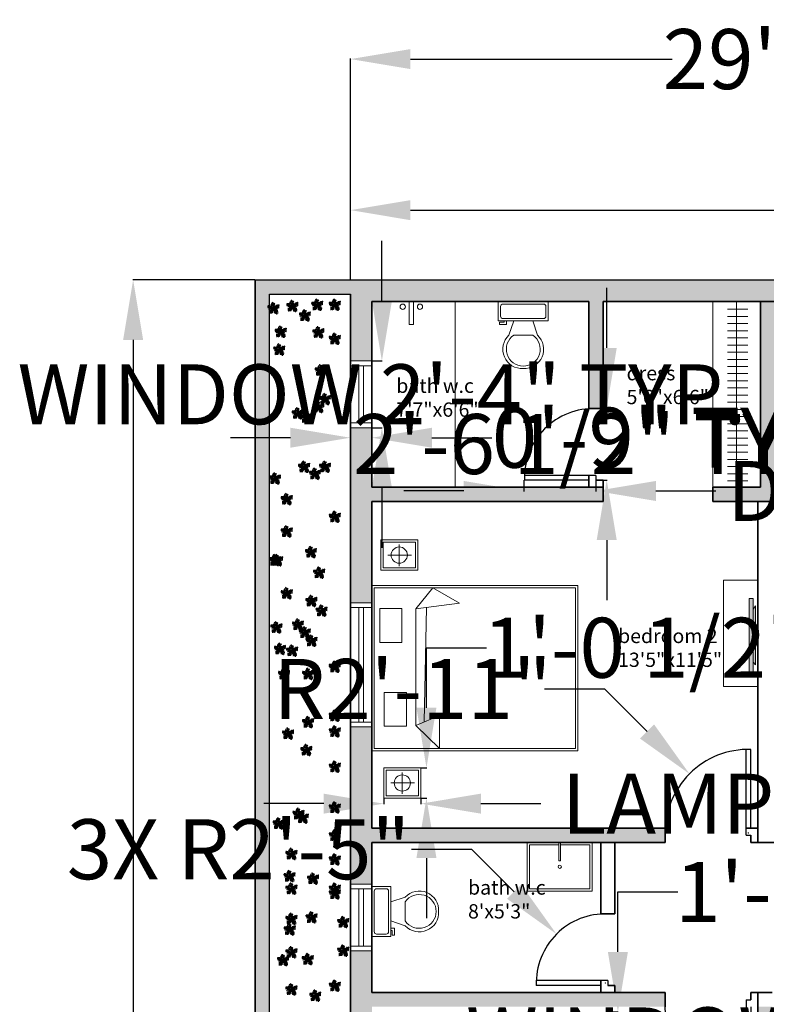
# Model space of a CAD drawing. Units: inches. Extents: x 23 to 3024, y 4 to 1405.
# Tile 2 of 7: x 2062 to 2375, y 992 to 1405. Entities that reach past the tile are written whole.
import ezdxf

# ---------------------------------------------------------------- set-up
doc = ezdxf.new("R2010")
doc.units = ezdxf.units.IN
doc.header["$MEASUREMENT"] = 0
for name, color, linetype, lineweight in [('A-ANNO-DIMS', 2, 'Continuous', 18), ('A-DOOR', 4, 'Continuous', 25), ('A-EQPM', 8, 'Continuous', 18), ('A-EQPM-PATT', 7, 'Continuous', 13), ('A-FLOR-CASE', 9, 'Continuous', 18), ('A-FLOR-FIXT', 9, 'Continuous', 18), ('A-WALL', 7, 'Continuous', 35), ('A-WALL-PATT', 189, 'Continuous', 13), ('C-PROP', 7, 'Continuous', 30), ('L-PLNT', 114, 'Continuous', 13)]:
    doc.layers.add(name, color=color, linetype=linetype, lineweight=lineweight)
for name, color, linetype, lineweight, true_color in [('A-AREA-IDEN', 30, 'Continuous', 18, 0xf8991e), ('A-FURN', 141, 'Continuous', 18, 0xadddf7), ('A-GLAZ', 30, 'Continuous', 18, 0xf26722)]:
    doc.layers.add(name, color=color, linetype=linetype, lineweight=lineweight, true_color=true_color)
doc.styles.get("Standard").update_dxf_attribs({"font": 'arial.ttf'})
doc.dimstyles.get("Standard").update_dxf_attribs({"dimtxt": 25.18, "dimasz": 25.18, "dimexe": 0.18, "dimexo": 0.0625, "dimgap": 0.09, "dimtad": 0, "dimtih": 1, "dimtoh": 1, "dimdec": 0, "dimrnd": 10, "dimzin": 0, "dimdsep": 46, "dimlunit": 3, "dimtxsty": 'Standard', "dimcen": 0.09, "dimadec": 0, "dimazin": 0, "dimtfac": 1, "dimtdec": 0, "dimtofl": 0, "dimtmove": 0, "dimatfit": 3, "dimfxl": 1, "dimtolj": 1, "dimtzin": 0, "dimarcsym": 0})

# ---------------------------------------------------------------- blocks, each defined once
blk = doc.blocks.new('*U2')
for p, q in [((9.5, -6), (9.5, -2)), ((-8, -8.5), (-8, -8)), ((-7, -8), (-7, -9.5)), ((-4, -8), (-6, -14)), ((4, -8), (6, -14)), ((-10, -8.5), (-8, -8.5)), ((-10, -9.5), (-10, -8.5)), ((-7, -9.5), (-10, -9.5)), ((4, -14), (-4, -14))]:
    blk.add_line(p, q)
blk.add_lwpolyline([(10.5, -8), (10.5, 0), (-10.5, 0), (-10.5, -8)], close=True)
for points in [[(-9.5, -2), (-9.5, -6)], [(8.5, -1), (-8.5, -1)], [(-8.5, -7), (8.5, -7)]]:
    blk.add_lwpolyline(points)
for centre, radius, start, end in [((-8.625, -1.875), 0.8839, 81.8699, 188.1301), ((8.625, -1.875), 0.8839, 351.8699, 98.1301), ((-8.625, -6.125), 0.8839, 171.869898, 278.1301), ((8.625, -6.125), 0.8839, 261.8699, 8.1301), ((-0.4772, -19.9188), 8.0953, 133.01722, 273.38), ((0.0374, -19.8731), 7.127, 124.50543, 269.7), ((-0.0373, -19.8731), 7.127, 270.3, 55.4946), ((0.4773, -19.9188), 8.0953, 266.62, 46.9828)]:
    blk.add_arc(centre, radius, start, end)
blk = doc.blocks.new('*U8')
for p, q in [((-47.498, 19.737), (-55.83, 18.344)), ((-40.615, 13.7), (-55.105, 10.913)), ((-31.5, 4.5), (-52.5, 25.5)), ((-33.37, 6.269), (-52.207, 5.34)), ((-48.585, 21.131), (-49.309, 29.026)), ((-28.299, 3.483), (-47.86, -5.805)), ((-43.513, 28.561), (-42.427, 15.558)), ((-38.442, 26.239), (-34.819, 7.663)), ((-21.416, 3.018), (-38.079, -8.128)), ((-35.544, 28.097), (-24.314, 3.947)), ((0, 0), (-31.5, 4.5)), ((-14.533, 2.09), (-30.834, 25.31)), ((-15.982, 2.09), (-30.11, -9.521)), ((-3.665, 19.273), (-27.574, 35.527)), ((-5.114, 28.097), (-24.676, 40.636)), ((-24.314, 23.917), (-2.941, 13.7)), ((0, 0), (-22.5, -19.5)), ((-7.288, 39.707), (-21.778, 46.673)), ((-6.563, 1.161), (-21.416, -8.128)), ((-20.691, 13.7), (-1.129, 4.876)), ((-8.737, 47.138), (-17.069, 52.711)), ((-10.186, 53.64), (-13.084, 55.962)), ((0, 0), (-10.5, 57)), ((-9.099, 51.782), (-6.563, 55.962)), ((-7.65, 43.423), (-2.578, 49.46)), ((-5.839, 35.992), (4.667, 48.067)), ((-5.114, 27.632), (10.463, 46.673)), ((-2.941, 16.486), (8.652, 37.85)), ((-1.129, 6.734), (9.014, 26.704)), ((0, 0), (27, 9)), ((0, 0), (18, -22.5)), ((3.942, 1.625), (11.187, 24.381)), ((6.478, 1.625), (26.04, -8.592)), ((10.101, 3.483), (17.708, 26.239)), ((11.187, 3.483), (30.749, -5.805)), ((16.259, 5.805), (23.142, 31.348)), ((18.07, 5.805), (35.096, -3.483)), ((22.055, 7.198), (27.489, 32.277)), ((24.229, 7.663), (46.688, 1.625)), ((27, 9), (48, 36)), ((27.127, 9.056), (31.112, 35.992)), ((29.662, 12.307), (48.137, 6.269)), ((31.836, 30.883), (32.561, 16.486)), ((33.285, 16.486), (48.862, 10.913)), ((35.096, 32.741), (37.27, 22.524)), ((36.183, 19.737), (48.137, 17.88)), ((38.719, 34.134), (41.979, 28.561)), ((40.53, 25.775), (48.862, 24.846)), ((43.791, 29.954), (51.036, 30.883)), ((44.153, 36.456), (45.239, 32.741)), ((-17.431, -15.094), (-42.789, -18.809)), ((-28.299, -29.026), (-42.789, -31.348)), ((-24.314, -21.596), (-42.427, -22.06)), ((-30.834, -34.135), (-42.427, -35.528)), ((-34.457, -39.708), (-40.978, -42.494)), ((-26.849, -26.24), (-40.253, -25.775)), ((-22.5, -19.5), (-37.5, -45)), ((-32.646, -36.921), (-31.921, -44.352)), ((-15.257, -12.772), (-30.11, -12.772)), ((-29.023, -30.884), (-27.936, -43.887)), ((-25.038, -23.918), (-22.865, -45.281)), ((-20.691, -18.345), (-17.793, -44.352)), ((-6.563, -5.805), (-19.967, -9.985)), ((-17.069, -15.094), (-12.721, -40.172)), ((-13.446, -11.378), (-8.737, -32.741)), ((-9.461, -8.592), (-6.201, -23.453)), ((-4.752, -3.483), (-3.665, -14.629)), ((2.493, -3.019), (-1.491, -20.202)), ((1.769, -2.555), (24.229, -9.521)), ((5.029, -6.27), (2.131, -25.775)), ((9.014, -11.378), (3.58, -35.992)), ((14.085, -16.951), (6.478, -40.172)), ((7.565, -9.056), (32.198, -14.629)), ((18.07, -22.524), (8.289, -45.745)), ((12.274, -15.094), (36.907, -18.809)), ((20.244, -30.419), (15.897, -44.816)), ((16.259, -19.738), (36.183, -22.989)), ((18, -22.5), (27, -52.5)), ((18.433, -22.524), (40.53, -29.026)), ((19.157, -25.311), (38.719, -33.206)), ((22.78, -37.85), (19.519, -48.532)), ((21.331, -32.741), (39.081, -40.636)), ((22.78, -38.314), (34.372, -44.816)), ((24.591, -45.745), (23.142, -50.854)), ((24.591, -43.423), (30.749, -47.603)), ((26.764, -49.925), (28.213, -50.854))]:
    blk.add_line(p, q)
blk = doc.blocks.new('*D9')
at = {"layer": 'A-ANNO-DIMS', "color": 0, "lineweight": -2, "transparency": 16777216}
for p, q in [((2200.45, 1295.99), (2200.45, 1325.4)), ((2225.63, 1325.22), (2478.99, 1325.22)), ((2775.27, 1325.22), (2521.91, 1325.22)), ((2800.45, 1295.99), (2800.45, 1325.4))]:
    blk.add_line(p, q, dxfattribs=at)
at = {"layer": 'A-ANNO-DIMS', "color": 0, "transparency": 16777216}
for points in [[(2225.63, 1329.42), (2225.63, 1321.02), (2200.45, 1325.22)], [(2775.27, 1329.42), (2775.27, 1321.02), (2800.45, 1325.22)]]:
    blk.add_solid(points, dxfattribs=at)
at = {"layer": 'Defpoints', "color": 0, "transparency": 16777216}
for p in [(2800.45, 1325.22), (2200.45, 1295.93), (2800.45, 1295.93)]:
    blk.add_point(p, dxfattribs=at)
at = {"layer": 'A-ANNO-DIMS', "color": 0, "transparency": 16777216, "insert": (2500.45, 1325.22), "char_height": 25.18, "attachment_point": 5}
blk.add_mtext("\\A1;50'", dxfattribs=at)
blk = doc.blocks.new('*D10')
at = {"layer": 'A-ANNO-DIMS', "color": 0, "lineweight": -2, "transparency": 16777216}
for p, q in [((2160.39, 1295.93), (2109.1, 1295.93)), ((2109.28, 1270.75), (2109.28, 948.87)), ((2109.28, 601.11), (2109.28, 922.98)), ((2160.39, 575.93), (2109.1, 575.93))]:
    blk.add_line(p, q, dxfattribs=at)
at = {"layer": 'A-ANNO-DIMS', "color": 0, "transparency": 16777216}
for points in [[(2105.08, 1270.75), (2113.48, 1270.75), (2109.28, 1295.93)], [(2105.08, 601.11), (2113.48, 601.11), (2109.28, 575.93)]]:
    blk.add_solid(points, dxfattribs=at)
at = {"layer": 'Defpoints', "color": 0, "transparency": 16777216}
for p in [(2160.45, 1295.93), (2109.28, 575.93), (2160.45, 575.93)]:
    blk.add_point(p, dxfattribs=at)
at = {"layer": 'A-ANNO-DIMS', "color": 0, "transparency": 16777216, "insert": (2109.28, 935.93), "char_height": 25.18, "attachment_point": 5}
blk.add_mtext("\\A1;60'", dxfattribs=at)
blk = doc.blocks.new('DOOR-SWING-36IN')
for p, q in [((-1, -1), (-1, 35)), ((1, 2), (1, 35)), ((-1, -1), (1, -1))]:
    blk.add_line(p, q)
blk.add_arc((0, 0), 35.01, 88.3634, 181.6366)
blk = doc.blocks.new('DOOR-SWING-30IN')
for p, q in [((1, 1), (-29, 1)), ((1, 1), (1, -1)), ((-2, -1), (-29, -1))]:
    blk.add_line(p, q)
blk.add_arc((0, 0), 29.02, 88.0251, 181.9749)
blk = doc.blocks.new('WINDOW-48IN')
for p, q in [((9, 52), (0, 52)), ((9, 50), (0, 50)), ((3.5, 2), (3.5, 50)), ((5.5, 2), (5.5, 50)), ((9, 2), (0, 2)), ((9, 0), (0, 0))]:
    blk.add_line(p, q)
blk = doc.blocks.new('WINDOW-24IN')
for p, q in [((9, 28), (0, 28)), ((9, 26), (0, 26)), ((3.5, 2), (3.5, 26)), ((5.5, 2), (5.5, 26)), ((9, 2), (0, 2)), ((9, 0), (0, 0))]:
    blk.add_line(p, q)
blk = doc.blocks.new('NIGHTSTAND-LAMP')
for p, q in [((7.79, 10.75), (7.79, 1.76)), ((2.95, 6.35), (12.92, 6.35))]:
    blk.add_line(p, q)
for points in [[(0, 12.71), (15.59, 12.71), (15.59, 0), (0, 0)], [(1, 11.71), (14.59, 11.71), (14.59, 1), (1, 1)]]:
    blk.add_lwpolyline(points, close=True)
blk.add_circle((7.79, 6.35), 3.4)
blk = doc.blocks.new('*D25')
at = {"layer": 'A-ANNO-DIMS', "color": 0, "lineweight": -2, "transparency": 16777216}
for p, q in [((2273.17, 1211.86), (2273.17, 1207.21)), ((2303.45, 1211.86), (2303.45, 1207.21)), ((2247.99, 1207.39), (2222.81, 1207.39)), ((2328.63, 1207.39), (2353.81, 1207.39))]:
    blk.add_line(p, q, dxfattribs=at)
at = {"layer": 'A-ANNO-DIMS', "color": 0, "transparency": 16777216}
for points in [[(2247.99, 1211.58), (2247.99, 1203.19), (2273.17, 1207.39)], [(2328.63, 1211.58), (2328.63, 1203.19), (2303.45, 1207.39)]]:
    blk.add_solid(points, dxfattribs=at)
at = {"layer": 'Defpoints', "color": 0, "transparency": 16777216}
for p in [(2273.17, 1211.93), (2303.45, 1211.93), (2303.45, 1207.39)]:
    blk.add_point(p, dxfattribs=at)
at = {"layer": 'A-ANNO-DIMS', "color": 0, "transparency": 16777216, "insert": (2517, 1207.39), "char_height": 25.18, "attachment_point": 5}
blk.add_mtext('\\A1;DOOR 2\'-6 1/2" TYP.', dxfattribs=at)
blk = doc.blocks.new('*D26')
at = {"layer": 'A-ANNO-DIMS', "color": 0, "lineweight": -2, "transparency": 16777216}
for p, q in [((2307.99, 1267.38), (2307.99, 1292.56)), ((2303.51, 1242.2), (2308.17, 1242.2)), ((2303.51, 1211.93), (2308.17, 1211.93)), ((2307.99, 1186.75), (2307.99, 1161.57))]:
    blk.add_line(p, q, dxfattribs=at)
at = {"layer": 'A-ANNO-DIMS', "color": 0, "transparency": 16777216}
for points in [[(2303.79, 1267.38), (2312.19, 1267.38), (2307.99, 1242.2)], [(2303.79, 1186.75), (2312.19, 1186.75), (2307.99, 1211.93)]]:
    blk.add_solid(points, dxfattribs=at)
at = {"layer": 'Defpoints', "color": 0, "transparency": 16777216}
for p in [(2303.45, 1242.2), (2307.99, 1242.2), (2303.45, 1211.93)]:
    blk.add_point(p, dxfattribs=at)
at = {"layer": 'A-ANNO-DIMS', "color": 0, "transparency": 16777216, "insert": (2307.99, 1227.07), "char_height": 25.18, "attachment_point": 5}
blk.add_mtext('\\A1;2\'-6 1/2" TYP.', dxfattribs=at)
blk = doc.blocks.new('*D27')
at = {"layer": 'A-ANNO-DIMS', "color": 0, "lineweight": -2, "transparency": 16777216}
for p, q in [((2217.25, 952.93), (2217.25, 978.11)), ((2217.25, 978.11), (2242.43, 978.11)), ((2209.51, 952.93), (2217.43, 952.93)), ((2217.25, 926.11), (2217.25, 927.75)), ((2209.51, 900.93), (2217.43, 900.93))]:
    blk.add_line(p, q, dxfattribs=at)
at = {"layer": 'A-ANNO-DIMS', "color": 0, "transparency": 16777216}
for points in [[(2213.05, 927.75), (2221.45, 927.75), (2217.25, 952.93)], [(2213.05, 926.11), (2221.45, 926.11), (2217.25, 900.93)]]:
    blk.add_solid(points, dxfattribs=at)
at = {"layer": 'Defpoints', "color": 0, "transparency": 16777216}
for p in [(2209.45, 952.93), (2217.25, 952.93), (2209.45, 900.93)]:
    blk.add_point(p, dxfattribs=at)
at = {"layer": 'A-ANNO-DIMS', "color": 0, "transparency": 16777216, "insert": (2401.83, 978.11), "char_height": 25.18, "attachment_point": 5}
blk.add_mtext('\\A1;WINDOW 4\'-4" TYP.', dxfattribs=at)
blk = doc.blocks.new('*D29')
at = {"layer": 'A-ANNO-DIMS', "color": 0, "lineweight": -2, "transparency": 16777216}
for p, q in [((2213.65, 1287.11), (2213.65, 1312.29)), ((2209.51, 1261.93), (2213.83, 1261.93)), ((2209.51, 1233.93), (2213.83, 1233.93)), ((2213.65, 1208.75), (2213.65, 1183.57))]:
    blk.add_line(p, q, dxfattribs=at)
at = {"layer": 'A-ANNO-DIMS', "color": 0, "transparency": 16777216}
for points in [[(2209.45, 1287.11), (2217.85, 1287.11), (2213.65, 1261.93)], [(2209.45, 1208.75), (2217.85, 1208.75), (2213.65, 1233.93)]]:
    blk.add_solid(points, dxfattribs=at)
at = {"layer": 'Defpoints', "color": 0, "transparency": 16777216}
for p in [(2209.45, 1261.93), (2213.65, 1261.93), (2209.45, 1233.93)]:
    blk.add_point(p, dxfattribs=at)
at = {"layer": 'A-ANNO-DIMS', "color": 0, "transparency": 16777216, "insert": (2213.65, 1247.93), "char_height": 25.18, "attachment_point": 5}
blk.add_mtext('\\A1;WINDOW 2\'-4" TYP.', dxfattribs=at)
blk = doc.blocks.new('*D30')
at = {"layer": 'A-ANNO-DIMS', "color": 0, "lineweight": -2, "transparency": 16777216}
for p, q in [((2200.45, 1233.86), (2200.45, 1229.55)), ((2209.45, 1233.86), (2209.45, 1229.55)), ((2175.27, 1229.73), (2150.09, 1229.73)), ((2234.63, 1229.73), (2259.81, 1229.73))]:
    blk.add_line(p, q, dxfattribs=at)
at = {"layer": 'A-ANNO-DIMS', "color": 0, "transparency": 16777216}
for points in [[(2175.27, 1233.92), (2175.27, 1225.53), (2200.45, 1229.73)], [(2234.63, 1233.92), (2234.63, 1225.53), (2209.45, 1229.73)]]:
    blk.add_solid(points, dxfattribs=at)
at = {"layer": 'Defpoints', "color": 0, "transparency": 16777216}
for p in [(2200.45, 1233.93), (2209.45, 1233.93), (2209.45, 1229.73)]:
    blk.add_point(p, dxfattribs=at)
at = {"layer": 'A-ANNO-DIMS', "color": 0, "transparency": 16777216, "insert": (2336.64, 1229.73), "char_height": 25.18, "attachment_point": 5}
blk.add_mtext('\\A1;0\'-9" TYP.', dxfattribs=at)
blk = doc.blocks.new('*D35')
at = {"layer": 'A-ANNO-DIMS', "color": 0, "lineweight": -2, "transparency": 16777216}
for p, q in [((2297.24, 975.85), (2297.24, 973.72)), ((2310.67, 975.85), (2310.67, 973.72)), ((2272.06, 973.9), (2246.88, 973.9)), ((2335.85, 973.9), (2361.03, 973.9))]:
    blk.add_line(p, q, dxfattribs=at)
at = {"layer": 'A-ANNO-DIMS', "color": 0, "transparency": 16777216}
for points in [[(2272.06, 978.09), (2272.06, 969.7), (2297.24, 973.9)], [(2335.85, 978.09), (2335.85, 969.7), (2310.67, 973.9)]]:
    blk.add_solid(points, dxfattribs=at)
at = {"layer": 'Defpoints', "color": 0, "transparency": 16777216}
for p in [(2297.24, 975.91), (2310.67, 975.91), (2310.67, 973.9)]:
    blk.add_point(p, dxfattribs=at)
at = {"layer": 'A-ANNO-DIMS', "color": 0, "transparency": 16777216, "insert": (2585.8, 973.9), "char_height": 25.18, "attachment_point": 5}
blk.add_mtext('\\A1;NIGHTSTAND 1\'-1 1/2" TYP.', dxfattribs=at)
blk = doc.blocks.new('*D36')
at = {"layer": 'A-ANNO-DIMS', "color": 0, "lineweight": -2, "transparency": 16777216}
for p, q in [((2312.68, 1013.98), (2312.68, 1039.16)), ((2312.68, 1039.16), (2337.86, 1039.16)), ((2310.73, 988.8), (2312.86, 988.8)), ((2310.73, 975.91), (2312.86, 975.91)), ((2312.68, 950.73), (2312.68, 925.55))]:
    blk.add_line(p, q, dxfattribs=at)
at = {"layer": 'A-ANNO-DIMS', "color": 0, "transparency": 16777216}
for points in [[(2308.48, 1013.98), (2316.88, 1013.98), (2312.68, 988.8)], [(2308.48, 950.73), (2316.88, 950.73), (2312.68, 975.91)]]:
    blk.add_solid(points, dxfattribs=at)
at = {"layer": 'Defpoints', "color": 0, "transparency": 16777216}
for p in [(2310.67, 988.8), (2312.68, 988.8), (2310.67, 975.91)]:
    blk.add_point(p, dxfattribs=at)
at = {"layer": 'A-ANNO-DIMS', "color": 0, "transparency": 16777216, "insert": (2413.51, 1039.16), "char_height": 25.18, "attachment_point": 5}
blk.add_mtext('\\A1;1\'-1" TYP.', dxfattribs=at)
blk = doc.blocks.new('*D37')
at = {"layer": 'A-ANNO-DIMS', "color": 0, "lineweight": -2, "transparency": 16777216}
for p, q in [((2214.42, 1078.46), (2214.42, 1076)), ((2230.01, 1078.46), (2230.01, 1076)), ((2189.24, 1076.18), (2164.06, 1076.18)), ((2255.19, 1076.18), (2280.37, 1076.18))]:
    blk.add_line(p, q, dxfattribs=at)
at = {"layer": 'A-ANNO-DIMS', "color": 0, "transparency": 16777216}
for points in [[(2189.24, 1080.38), (2189.24, 1071.99), (2214.42, 1076.18)], [(2255.19, 1080.38), (2255.19, 1071.99), (2230.01, 1076.18)]]:
    blk.add_solid(points, dxfattribs=at)
at = {"layer": 'Defpoints', "color": 0, "transparency": 16777216}
for p in [(2214.42, 1078.52), (2230.01, 1078.52), (2230.01, 1076.18)]:
    blk.add_point(p, dxfattribs=at)
at = {"layer": 'A-ANNO-DIMS', "color": 0, "transparency": 16777216, "insert": (2499.37, 1076.18), "char_height": 25.18, "attachment_point": 5}
blk.add_mtext('\\A1;LAMP TABLE 1\'-3 1/2" TYP.', dxfattribs=at)
blk = doc.blocks.new('*D38')
at = {"layer": 'A-ANNO-DIMS', "color": 0, "lineweight": -2, "transparency": 16777216}
for p, q in [((2232.35, 1116.41), (2232.35, 1141.59)), ((2232.35, 1141.59), (2257.53, 1141.59)), ((2230.07, 1091.23), (2232.53, 1091.23)), ((2230.07, 1078.52), (2232.53, 1078.52)), ((2232.35, 1053.34), (2232.35, 1028.16))]:
    blk.add_line(p, q, dxfattribs=at)
at = {"layer": 'A-ANNO-DIMS', "color": 0, "transparency": 16777216}
for points in [[(2228.15, 1116.41), (2236.54, 1116.41), (2232.35, 1091.23)], [(2228.15, 1053.34), (2236.54, 1053.34), (2232.35, 1078.52)]]:
    blk.add_solid(points, dxfattribs=at)
at = {"layer": 'Defpoints', "color": 0, "transparency": 16777216}
for p in [(2230.01, 1091.23), (2232.35, 1091.23), (2230.01, 1078.52)]:
    blk.add_point(p, dxfattribs=at)
at = {"layer": 'A-ANNO-DIMS', "color": 0, "transparency": 16777216, "insert": (2362.51, 1141.59), "char_height": 25.18, "attachment_point": 5}
blk.add_mtext('\\A1;1\'-0 1/2" TYP.', dxfattribs=at)
blk = doc.blocks.new('*D44')
at = {"layer": 'A-ANNO-DIMS', "color": 0, "lineweight": -2, "transparency": 16777216}
for p, q in [((2200.45, 1295.99), (2200.45, 1388.79)), ((2225.63, 1388.61), (2335.4, 1388.61)), ((2532.27, 1388.61), (2422.5, 1388.61)), ((2557.45, 1286.99), (2557.45, 1388.79))]:
    blk.add_line(p, q, dxfattribs=at)
at = {"layer": 'A-ANNO-DIMS', "color": 0, "transparency": 16777216}
for points in [[(2225.63, 1392.81), (2225.63, 1384.42), (2200.45, 1388.61)], [(2532.27, 1392.81), (2532.27, 1384.42), (2557.45, 1388.61)]]:
    blk.add_solid(points, dxfattribs=at)
at = {"layer": 'Defpoints', "color": 0, "transparency": 16777216}
for p in [(2557.45, 1388.61), (2200.45, 1295.93), (2557.45, 1286.93)]:
    blk.add_point(p, dxfattribs=at)
at = {"layer": 'A-ANNO-DIMS', "color": 0, "transparency": 16777216, "insert": (2378.95, 1388.61), "char_height": 25.18, "attachment_point": 5}
blk.add_mtext('\\A1;29\'-9"', dxfattribs=at)
blk = doc.blocks.new('*D48')
at = {"layer": 'A-ANNO-DIMS', "color": 0, "lineweight": -2, "transparency": 16777216}
for p, q in [((2281.9, 1124.3), (2307.08, 1124.3)), ((2307.08, 1124.3), (2324.89, 1106.49)), ((2367.36, 1063.93), (2367.54, 1063.93)), ((2367.45, 1063.84), (2367.45, 1064.02))]:
    blk.add_line(p, q, dxfattribs=at)
at = {"layer": 'A-ANNO-DIMS', "color": 0, "transparency": 16777216}
blk.add_solid([(2327.85, 1109.46), (2321.92, 1103.52), (2342.69, 1088.69)], dxfattribs=at)
at = {"layer": 'Defpoints', "color": 0, "transparency": 16777216}
for p in [(2342.69, 1088.69), (2367.45, 1063.93)]:
    blk.add_point(p, dxfattribs=at)
at = {"layer": 'A-ANNO-DIMS', "color": 0, "transparency": 16777216, "insert": (2226.51, 1124.3), "char_height": 25.18, "attachment_point": 5}
blk.add_mtext('\\A1;R2\'-11"', dxfattribs=at)
blk = doc.blocks.new('*D49')
at = {"layer": 'A-ANNO-DIMS', "color": 0, "lineweight": -2, "transparency": 16777216}
for p, q in [((2226.14, 1057.06), (2251.32, 1057.06)), ((2251.32, 1057.06), (2269.13, 1039.25)), ((2307.36, 1000.93), (2307.54, 1000.93)), ((2307.45, 1000.84), (2307.45, 1001.02))]:
    blk.add_line(p, q, dxfattribs=at)
at = {"layer": 'A-ANNO-DIMS', "color": 0, "transparency": 16777216}
blk.add_solid([(2272.09, 1042.22), (2266.16, 1036.28), (2286.93, 1021.45)], dxfattribs=at)
at = {"layer": 'Defpoints', "color": 0, "transparency": 16777216}
for p in [(2286.93, 1021.45), (2307.45, 1000.93)]:
    blk.add_point(p, dxfattribs=at)
at = {"layer": 'A-ANNO-DIMS', "color": 0, "transparency": 16777216, "insert": (2153.49, 1057.06), "char_height": 25.18, "attachment_point": 5}
blk.add_mtext('\\A1;3X R2\'-5"', dxfattribs=at)

msp = doc.modelspace()

# ---------------------------------------------------------------- hatches: boundary and pattern name
at = {"layer": 'A-EQPM-PATT'}
h = msp.add_hatch(color=256, dxfattribs=at)
h.dxf.hatch_style = 1
h.paths.add_polyline_path([(2566.39, 889.19), (2562.89, 889.19), (2562.89, 848.35), (2566.39, 848.35)])
h.paths.add_polyline_path([(2562.89, 883.28), (2559.32, 885.34), (2559.32, 851.44), (2562.89, 854.81)])
h.paths.add_polyline_path([(2370.36, 1159.16), (2369.43, 1157.81), (2369.43, 1135.58), (2370.36, 1134.43)])
h.paths.add_polyline_path([(2369.43, 1162.31), (2367.73, 1162.31), (2367.73, 1131.3), (2369.43, 1131.3)])
h.paths.add_polyline_path([(2381.34, 1160.62), (2379.7, 1162.16), (2380.08, 1134.79), (2381.34, 1136.43)])
h.paths.add_polyline_path([(2383.55, 1164.18), (2381.34, 1164.18), (2381.34, 1130.16), (2383.55, 1130.16)])
at = {"layer": 'A-WALL-PATT'}
h = msp.add_hatch(color=256, dxfattribs=at)
h.dxf.hatch_style = 1
h.paths.add_polyline_path([(2209.45, 1233.93), (2200.45, 1233.93), (2200.45, 1160.43), (2209.45, 1160.43), (2209.45, 1167.77), (2209.45, 1202.93), (2306.45, 1202.93), (2306.45, 1208.93), (2300.45, 1208.93), (2209.45, 1208.93)], flags=17)
h.paths.add_polyline_path([(2800.45, 1295.93), (2200.45, 1295.93), (2160.45, 1295.93), (2160.45, 575.93), (2200.45, 575.93), (2228.06, 575.93), (2228.06, 584.93), (2209.45, 584.93), (2209.45, 856.93), (2200.45, 856.93), (2200.45, 581.93), (2166.45, 581.93), (2166.45, 1289.93), (2200.45, 1289.93), (2200.45, 1261.93), (2209.45, 1261.93), (2209.45, 1286.93), (2244.45, 1286.93), (2300.45, 1286.93), (2300.45, 1241.93), (2301.45, 1241.93, -0.017236), (2303.45, 1241.93), (2306.45, 1241.93), (2306.45, 1286.93), (2548.45, 1286.93), (2548.45, 1261.93), (2557.45, 1261.93), (2557.45, 1286.93), (2791.45, 1286.93), (2791.45, 1140.93), (2613.74, 1140.93), (2613.74, 1134.93), (2791.45, 1134.93), (2791.45, 927.1), (2800.45, 927.1)])
h.paths.add_polyline_path([(2166.06, 1284.53), (2166.03, 1284.87), (2166.29, 1284.91), (2166.32, 1284.58)], flags=16)
h.paths.add_polyline_path([(2557.45, 1233.93), (2548.45, 1233.93), (2548.45, 1208.93), (2514.78, 1208.93), (2457.45, 1208.93), (2451.45, 1208.93), (2451.45, 1202.93), (2548.45, 1202.93), (2557.45, 1202.93)], flags=17)
h.paths.add_polyline_path([(2457.45, 1286.93), (2451.45, 1286.93), (2451.45, 1241.93), (2454.45, 1241.93, -0.017236), (2456.45, 1241.93), (2457.45, 1241.93)], flags=17)
h.paths.add_polyline_path([(2419.96, 1208.93), (2378.45, 1208.93), (2378.45, 1286.93), (2372.45, 1286.93), (2372.45, 1208.93), (2352.45, 1208.93), (2352.45, 1202.93), (2419.96, 1202.93)], flags=17)
h.paths.add_polyline_path([(2557.45, 1134.93), (2563.84, 1134.93), (2563.84, 1140.93), (2557.45, 1140.93), (2557.45, 1149.12), (2548.45, 1149.12), (2548.45, 1103.07), (2548.45, 1065.93), (2416.45, 1065.93), (2416.45, 1064.93, -0.014283), (2416.45, 1062.93), (2416.45, 1059.93), (2548.45, 1059.93), (2548.45, 1025.12), (2557.45, 1025.12)], flags=17)
h.paths.add_polyline_path([(2332.45, 1062.93, -0.014283), (2332.45, 1064.93), (2332.45, 1065.93), (2209.45, 1065.93), (2209.45, 1108.43), (2200.45, 1108.43), (2200.45, 1042.43), (2209.45, 1042.43), (2209.45, 1059.93), (2332.45, 1059.93)], flags=17)
h.paths.add_polyline_path([(2332.45, 996.93), (2209.45, 996.93), (2209.45, 1014.43), (2200.45, 1014.43), (2200.45, 952.93), (2209.45, 952.93), (2209.45, 990.93), (2332.45, 990.93), (2332.45, 991.93, -0.014283), (2332.45, 993.93)], flags=17)
h.paths.add_polyline_path([(2209.45, 900.93), (2200.45, 900.93), (2200.45, 856.93), (2209.45, 856.93), (2255.95, 856.93), (2255.95, 862.93), (2209.45, 862.93)], flags=17)
h.paths.add_polyline_path([(2377.45, 823.93), (2374.45, 823.93, -0.017236), (2372.45, 823.93), (2371.45, 823.93), (2371.45, 763.93), (2312.45, 763.93), (2312.45, 791.27), (2312.45, 796.43), (2306.45, 796.43), (2306.45, 757.93), (2436.95, 757.93), (2436.95, 763.93), (2377.45, 763.93)], flags=17)
h.paths.add_polyline_path([(2557.45, 948.81), (2548.45, 948.81), (2548.45, 763.93), (2488.95, 763.93), (2488.95, 757.93), (2560.45, 757.93), (2560.45, 760.93), (2562.45, 760.93), (2562.45, 763.93), (2557.45, 763.93)], flags=17)
h.paths.add_polyline_path([(2377.45, 990.93), (2371.45, 990.93), (2371.45, 862.93), (2306.45, 862.93), (2306.45, 856.93), (2306.45, 824.43), (2312.45, 824.43), (2312.45, 856.93), (2371.45, 856.93), (2377.45, 856.93)], flags=17)
h.paths.add_polyline_path([(2800.45, 875.1), (2791.45, 875.1), (2791.45, 763.93), (2719.93, 763.93), (2719.93, 757.93), (2791.45, 757.93), (2791.45, 584.93), (2338.88, 584.93), (2338.88, 575.93), (2800.45, 575.93)], flags=17)
h.paths.add_polyline_path([(2667.93, 763.93), (2596.45, 763.93), (2596.45, 762.93, -0.014283), (2596.45, 760.93), (2596.45, 757.93), (2667.93, 757.93)], flags=16)

# ---------------------------------------------------------------- linework, layer by layer
at = {"layer": 'A-EQPM'}
for p, q in [((2369.43, 1157.81), (2370.36, 1159.16)), ((2370.36, 1159.16), (2370.36, 1134.43)), ((2370.36, 1134.43), (2369.43, 1135.58))]:
    msp.add_line(p, q, dxfattribs=at)
for points in [[(2371.45, 1169.9), (2356.95, 1169.9), (2356.95, 1125.3), (2371.45, 1125.3)], [(2369.43, 1162.31), (2367.73, 1162.31), (2367.73, 1131.3), (2369.43, 1131.3)]]:
    msp.add_lwpolyline(points, close=True, dxfattribs=at)
at = {"layer": 'A-FLOR-CASE'}
for p, q in [((2362.45, 1286.93), (2362.45, 1208.93)), ((2358.68, 1283.61), (2367.22, 1283.61)), ((2358.68, 1280.61), (2367.22, 1280.61)), ((2358.68, 1277.61), (2367.22, 1277.61)), ((2358.68, 1274.61), (2367.22, 1274.61)), ((2358.68, 1271.61), (2367.22, 1271.61)), ((2358.68, 1268.61), (2367.22, 1268.61)), ((2358.68, 1265.61), (2367.22, 1265.61)), ((2358.68, 1262.61), (2367.22, 1262.61)), ((2358.68, 1259.61), (2367.22, 1259.61)), ((2358.68, 1256.61), (2367.22, 1256.61)), ((2358.68, 1253.61), (2367.22, 1253.61)), ((2358.68, 1250.61), (2367.22, 1250.61)), ((2358.68, 1247.61), (2367.22, 1247.61)), ((2358.68, 1244.61), (2367.22, 1244.61)), ((2358.68, 1241.61), (2367.22, 1241.61)), ((2358.68, 1238.61), (2367.22, 1238.61)), ((2358.68, 1235.61), (2367.22, 1235.61)), ((2358.68, 1232.61), (2367.22, 1232.61)), ((2358.68, 1229.61), (2367.22, 1229.61)), ((2358.68, 1226.61), (2367.22, 1226.61)), ((2358.68, 1223.61), (2367.22, 1223.61)), ((2358.68, 1220.61), (2367.22, 1220.61)), ((2358.68, 1217.61), (2367.22, 1217.61)), ((2358.68, 1214.61), (2367.22, 1214.61)), ((2358.68, 1211.61), (2367.22, 1211.61))]:
    msp.add_line(p, q, dxfattribs=at)
msp.add_lwpolyline([(2372.45, 1286.93), (2352.45, 1286.93), (2352.45, 1208.93), (2372.45, 1208.93)], close=True, dxfattribs=at)
at = {"layer": 'A-FLOR-FIXT'}
for points in [[(2209.45, 1286.93), (2244.45, 1286.93), (2244.45, 1208.93), (2209.45, 1208.93)], [(2226.95, 1286.93), (2225.08, 1286.93), (2225.08, 1277.27), (2226.95, 1277.27)], [(2274.55, 1059.93), (2301.94, 1059.93), (2301.94, 1039.5), (2274.55, 1039.5)], [(2288.61, 1059.93), (2287.88, 1059.93), (2287.88, 1052.19), (2288.61, 1052.19)]]:
    msp.add_lwpolyline(points, close=True, dxfattribs=at)
msp.add_lwpolyline([(2288.61, 1058.93), (2300.94, 1058.93), (2300.94, 1040.5), (2275.55, 1040.5), (2275.55, 1058.93), (2287.88, 1058.93)], dxfattribs=at)
for centre, radius in [((2222.39, 1284.69), 1.1), ((2229.63, 1284.69), 1.1), ((2288.25, 1049.71), 0.697)]:
    msp.add_circle(centre, radius, dxfattribs=at)
at = {"layer": 'A-FURN'}
for p, q in [((2227.93, 1158), (2235.02, 1166.77)), ((2235.02, 1166.77), (2246.25, 1160.29)), ((2246.25, 1160.29), (2227.93, 1158)), ((2227.93, 1158), (2227.93, 1109.02)), ((2232.33, 1158.55), (2231.43, 1110.48)), ((2237.81, 1113.15), (2227.93, 1109.02)), ((2237.81, 1099.34), (2237.81, 1113.15)), ((2227.93, 1109.02), (2237.81, 1099.34))]:
    msp.add_line(p, q, dxfattribs=at)
for points in [[(2209.45, 1167.77), (2295.93, 1167.77), (2295.93, 1098.34), (2209.45, 1098.34)], [(2210.45, 1166.77), (2294.93, 1166.77), (2294.93, 1099.34), (2210.45, 1099.34)], [(2222.08, 1158.06), (2212.75, 1158.06), (2212.75, 1143.83), (2222.08, 1143.83)], [(2223.95, 1122.88), (2214.61, 1122.88), (2214.61, 1108.65), (2223.95, 1108.65)]]:
    msp.add_lwpolyline(points, close=True, dxfattribs=at)
at = {"layer": 'A-WALL'}
for p, q in [((2200.45, 581.93), (2200.45, 1289.93)), ((2209.45, 1286.93), (2300.45, 1286.93)), ((2209.45, 1208.93), (2209.45, 1286.93)), ((2300.45, 1241.88), (2300.45, 1286.93)), ((2306.45, 1286.93), (2548.45, 1286.93)), ((2306.45, 1241.93), (2306.45, 1286.93)), ((2372.45, 1208.93), (2372.45, 1286.93)), ((2300.45, 1241.93), (2306.45, 1241.93)), ((2300.45, 1208.93), (2300.45, 1213.93)), ((2303.45, 1211.93), (2306.45, 1211.93)), ((2306.45, 1208.93), (2306.45, 1211.93)), ((2209.45, 1208.93), (2300.45, 1208.93)), ((2300.45, 1208.93), (2306.45, 1208.93)), ((2306.45, 1208.93), (2306.45, 1202.93)), ((2352.45, 1208.93), (2372.45, 1208.93)), ((2352.45, 1208.93), (2352.45, 1202.93)), ((2209.45, 1202.93), (2306.45, 1202.93)), ((2209.45, 1065.93), (2209.45, 1202.93)), ((2352.45, 1202.93), (2419.96, 1202.93)), ((2371.45, 1065.93), (2371.45, 1202.93)), ((2209.45, 1065.93), (2332.49, 1065.93)), ((2332.45, 1065.93), (2332.45, 1059.93)), ((2366.45, 1065.93), (2371.45, 1065.93)), ((2371.45, 1065.93), (2371.45, 1059.93)), ((2368.45, 1062.93), (2368.45, 1059.93)), ((2209.45, 1059.93), (2332.45, 1059.93)), ((2209.45, 996.93), (2209.45, 1059.93)), ((2305.45, 1029.88), (2305.45, 1059.93)), ((2311.45, 1029.93), (2311.45, 1059.93)), ((2368.45, 1059.93), (2380.45, 1059.93)), ((2305.45, 1029.93), (2311.45, 1029.93)), ((2305.45, 996.93), (2305.45, 1001.93)), ((2308.45, 999.93), (2311.45, 999.93)), ((2311.45, 996.93), (2311.45, 999.93)), ((2209.45, 996.93), (2332.45, 996.93)), ((2332.45, 996.93), (2332.45, 990.93)), ((2368.45, 996.93), (2368.45, 993.93)), ((2368.45, 996.93), (2377.45, 996.93)), ((2371.45, 996.93), (2371.45, 862.93))]:
    msp.add_line(p, q, dxfattribs=at)
at = {"layer": 'C-PROP'}
for p, q in [((2160.45, 575.93), (2160.45, 1295.93)), ((2160.45, 1295.93), (2200.45, 1295.93)), ((2160.45, 1295.93), (2160.45, 575.93)), ((2200.45, 1295.93), (2800.45, 1295.93)), ((2166.45, 1289.93), (2200.45, 1289.93)), ((2166.45, 581.93), (2166.45, 1289.93))]:
    msp.add_line(p, q, dxfattribs=at)

# ---------------------------------------------------------------- block references
at = {"layer": 'A-DOOR'}
for name, p in [('DOOR-SWING-30IN', (2302.45, 1212.93)), ('DOOR-SWING-36IN', (2367.45, 1063.93)), ('DOOR-SWING-30IN', (2307.45, 1000.93))]:
    msp.add_blockref(name, p, dxfattribs=at)
at = {"layer": 'A-DOOR', "extrusion": (0, 0, -1), "zscale": -1, "rotation": 180}
msp.add_blockref('DOOR-SWING-36IN', (-2367.45, 992.93), dxfattribs=at)
at = {"layer": 'A-FLOR-FIXT'}
msp.add_blockref('*U2', (2272.97, 1286.76), dxfattribs=at)
at = {"layer": 'A-FLOR-FIXT', "rotation": 90}
msp.add_blockref('*U2', (2209.45, 1030.97), dxfattribs=at)
at = {"layer": 'A-FURN'}
for p in [(2213.15, 1174.13), (2214.42, 1078.52)]:
    msp.add_blockref('NIGHTSTAND-LAMP', p, dxfattribs=at)
at = {"layer": 'A-GLAZ'}
for name, p in [('WINDOW-24IN', (2200.45, 1233.93)), ('WINDOW-48IN', (2200.45, 1108.43)), ('WINDOW-24IN', (2200.45, 1014.43))]:
    msp.add_blockref(name, p, dxfattribs=at)
at = {"layer": 'L-PLNT', "xscale": 0.0466330202614855, "yscale": 0.0466330202614855, "zscale": 0.0466330202614855}
for p in [(2168.29, 1283.95), (2176.21, 1284.88), (2186.64, 1285.4), (2194.03, 1285.4), (2181.48, 1280.91), (2171.33, 1274.07), (2187.12, 1273.83), (2194.03, 1271.1), (2170.7, 1266.59), (2188.09, 1257.91), (2189.91, 1245.83), (2187.12, 1242.48), (2178.45, 1239.84), (2182.14, 1238.21), (2181.13, 1217.41), (2189.91, 1217.44), (2168.9, 1212.5), (2185.67, 1214.5), (2173.84, 1203.86), (2194.03, 1196.45), (2173.84, 1190.28), (2184, 1181.63), (2168.88, 1178.24), (2169.84, 1178.19), (2187.44, 1173), (2173.84, 1164.35), (2184.18, 1161.12), (2188.46, 1157.03), (2178.54, 1151.2), (2169.52, 1150.02), (2181.46, 1147.9), (2184.25, 1144.41), (2171.02, 1141.01), (2176.08, 1140.27), (2172.69, 1130.51), (2182.83, 1130.51), (2194.03, 1133.49), (2194.03, 1112.94), (2182.83, 1110.26), (2174.39, 1105.47), (2194.03, 1106.38), (2182.05, 1098.58), (2194.03, 1091.57), (2178.79, 1071.77), (2194.03, 1074.44), (2170.46, 1067.74), (2180.55, 1070.22), (2194.03, 1062.75), (2175.81, 1054.97), (2194.03, 1052.63), (2175.03, 1045.62), (2184.88, 1044.61), (2175.81, 1040.38), (2194.03, 1040.38), (2194.03, 1038.38), (2175.81, 1027.71), (2184.26, 1028.34), (2197.53, 1026.38), (2175.1, 1023.28), (2175.81, 1013.69), (2197.53, 1014.38), (2172.35, 1010.39), (2182.69, 1010.83), (2175.81, 998.12), (2194.03, 999.67), (2185.82, 995.5)]:
    msp.add_blockref('*U8', p, dxfattribs=at)

# ---------------------------------------------------------------- texts
at = {"layer": 'A-AREA-IDEN', "char_height": 6, "attachment_point": 1}
for s, insert in [('dress \\P5\'6"x6\'6"', (2316.33, 1259.82)), ('bath w.c\\P7\'7"x6\'6" ', (2219.69, 1254.54)), ('bedroom 2\\P13\'5"x11\'5"', (2312.77, 1149.56)), ('bath w.c\\P8\'x5\'3"', (2249.8, 1044))]:
    msp.add_mtext_dynamic_manual_height_columns(s, width=46.8839, gutter_width=1, heights=[0], dxfattribs=dict(at, insert=insert))

# ---------------------------------------------------------------- dimensions: what is measured, and where the dimension line sits
at = {"layer": 'A-ANNO-DIMS'}
for base, p2, override, picture, middle in [((2557.45, 1388.61), (2557.45, 1286.93), {"dimdec": 1, "dimlfac": 1, "dimrnd": 0, "dimzin": 1, "dimdsep": 46, "dimlunit": 4, "dimfrac": 2}, '*D44', (2378.95, 1388.61)), ((2800.45, 1325.22), (2800.45, 1295.93), {"dimclrd": 0, "dimclre": 0, "dimclrt": 0}, '*D9', (2500.45, 1325.22))]:
    dim = msp.add_linear_dim(base=base, p1=(2200.45, 1295.93), p2=p2, dimstyle='Standard', override=override, dxfattribs=at)
    dim.commit()
    dim.dimension.update_dxf_attribs({"geometry": picture, "text_midpoint": middle})
for base, p1, p2, text, picture, middle in [((2213.65, 1261.93), (2209.45, 1233.93), (2209.45, 1261.93), 'WINDOW <> TYP.', '*D29', (2213.65, 1247.93)), ((2307.99, 1242.2), (2303.45, 1211.93), (2303.45, 1242.2), '<> TYP.', '*D26', (2307.99, 1227.07)), ((2232.35, 1091.23), (2230.01, 1078.52), (2230.01, 1091.23), '<> TYP.', '*D38', (2362.51, 1141.59)), ((2312.68, 988.8), (2310.67, 975.91), (2310.67, 988.8), '<> TYP.', '*D36', (2413.51, 1039.16)), ((2217.25, 952.93), (2209.45, 900.93), (2209.45, 952.93), 'WINDOW <> TYP.', '*D27', (2401.83, 978.11))]:
    dim = msp.add_linear_dim(base=base, p1=p1, p2=p2, angle=90, text=text, dimstyle='Standard', override={"dimdec": 1, "dimlfac": 1, "dimrnd": 0, "dimzin": 1, "dimdsep": 46, "dimlunit": 4, "dimfrac": 2}, dxfattribs=at)
    dim.commit()
    dim.dimension.update_dxf_attribs({"geometry": picture, "text_midpoint": middle})
dim = msp.add_linear_dim(base=(2109.28, 575.93), p1=(2160.45, 1295.93), p2=(2160.45, 575.93), angle=90, dimstyle='Standard', override={"dimclrd": 0, "dimclre": 0, "dimclrt": 0}, dxfattribs=at)
dim.commit()
dim.dimension.update_dxf_attribs({"geometry": '*D10', "text_midpoint": (2109.28, 935.93)})
for base, p1, p2, text, picture, middle in [((2303.45, 1207.39), (2273.17, 1211.93), (2303.45, 1211.93), 'DOOR <> TYP.', '*D25', (2517, 1207.39)), ((2209.45, 1229.73), (2200.45, 1233.93), (2209.45, 1233.93), '<> TYP.', '*D30', (2336.64, 1229.73)), ((2230.01, 1076.18), (2214.42, 1078.52), (2230.01, 1078.52), 'LAMP TABLE <> TYP.', '*D37', (2499.37, 1076.18)), ((2310.67, 973.9), (2297.24, 975.91), (2310.67, 975.91), 'NIGHTSTAND <> TYP.', '*D35', (2585.8, 973.9))]:
    dim = msp.add_linear_dim(base=base, p1=p1, p2=p2, text=text, dimstyle='Standard', override={"dimdec": 1, "dimlfac": 1, "dimrnd": 0, "dimzin": 1, "dimdsep": 46, "dimlunit": 4, "dimfrac": 2}, dxfattribs=at)
    dim.commit()
    dim.dimension.update_dxf_attribs({"geometry": picture, "text_midpoint": middle})
dim = msp.add_radius_dim(center=(2367.45, 1063.93), mpoint=(2342.69, 1088.69), dimstyle='Standard', override={"dimdec": 1, "dimlfac": 1, "dimrnd": 0, "dimzin": 1, "dimdsep": 46, "dimlunit": 4, "dimfrac": 2}, dxfattribs=at)
dim.commit()
dim.dimension.update_dxf_attribs({"geometry": '*D48', "text_midpoint": (2226.51, 1124.3)})
dim = msp.add_radius_dim(center=(2307.45, 1000.93), mpoint=(2286.93, 1021.45), text='3X <>', dimstyle='Standard', override={"dimdec": 1, "dimlfac": 1, "dimrnd": 0, "dimzin": 1, "dimdsep": 46, "dimlunit": 4, "dimfrac": 2}, dxfattribs=at)
dim.commit()
dim.dimension.update_dxf_attribs({"geometry": '*D49', "text_midpoint": (2153.49, 1057.06)})

doc.saveas('drawing.dxf')
